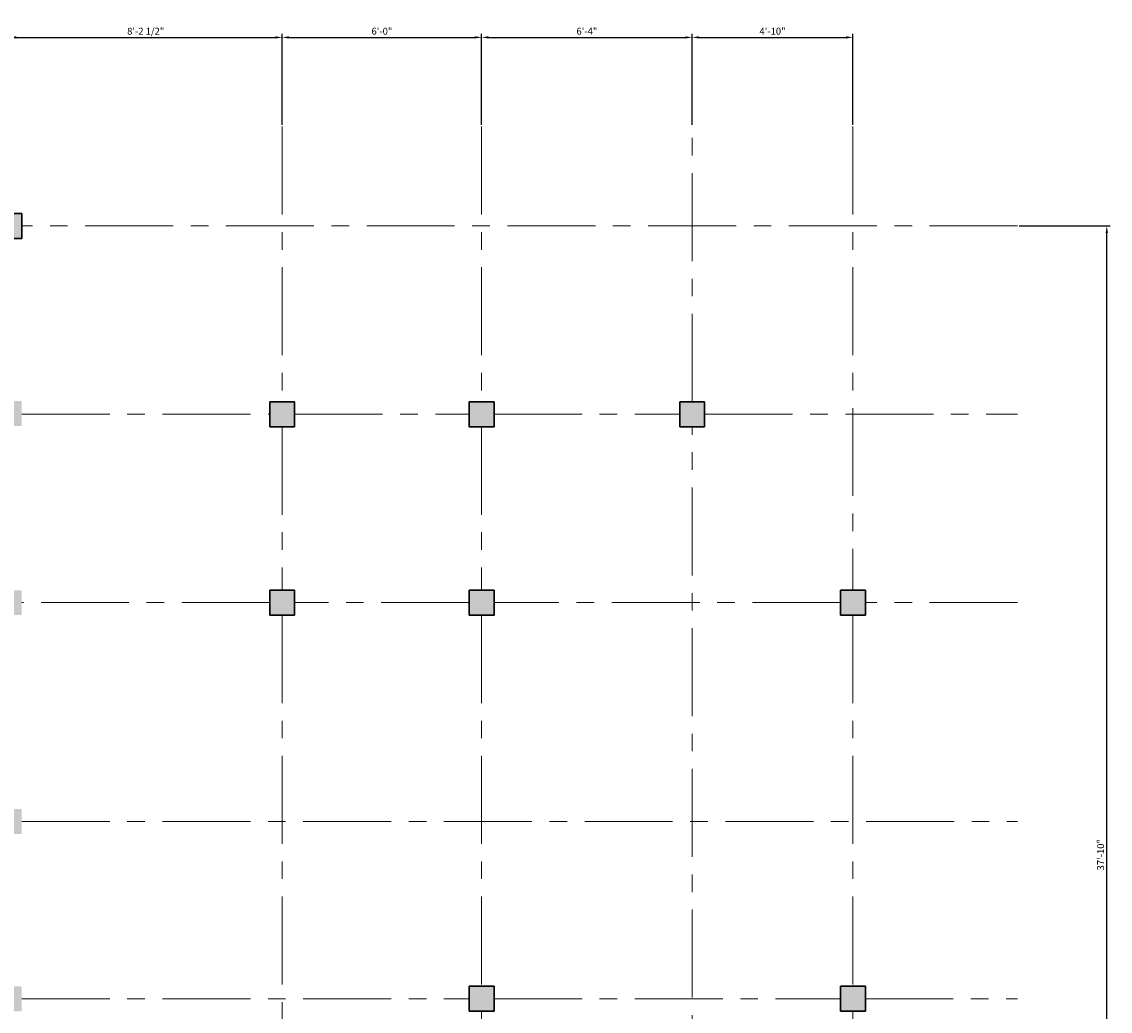
# Model space of a CAD drawing. Units: inches. Extents: x 4878 to 9282, y 5367 to 6617.
# Tile 9 of 14: x 5718 to 6111, y 6031 to 6388. Entities that reach past the tile are written whole.
import ezdxf

# ---------------------------------------------------------------- set-up
doc = ezdxf.new("R2010")
doc.units = ezdxf.units.IN
doc.linetypes.add('CENTER', pattern=[50.8, 31.75, -6.35, 6.35, -6.35])
for name, color, linetype, lineweight in [('A-ANNO-DIMS', 2, 'Continuous', 18), ('S-COLS', 1, 'Continuous', 30), ('S-COLS-PATT', 1, 'Continuous', 13), ('S-GRID', 4, 'CENTER', 13)]:
    doc.layers.add(name, color=color, linetype=linetype, lineweight=lineweight)
doc.styles.get("Standard").update_dxf_attribs({"font": 'arial.ttf'})
doc.dimstyles.new('ISO-25', dxfattribs={"dimtxt": 2.5, "dimasz": 2.5, "dimexe": 1.25, "dimexo": 0.625, "dimtad": 1, "dimdec": 0, "dimlunit": 3, "dimtxsty": 'Standard', "dimcen": 2.5, "dimadec": 0, "dimazin": 0, "dimtfac": 1, "dimtdec": 0, "dimtmove": 0, "dimatfit": 3, "dimfxl": 1, "dimarcsym": 0})

# ---------------------------------------------------------------- blocks, each defined once
blk = doc.blocks.new('COLUMN-9X9')
for p, q in [((0, 9), (9, 9)), ((0, 0), (0, 9)), ((9, 9), (9, 0)), ((0, 0), (9, 0))]:
    blk.add_line(p, q)
blk = doc.blocks.new('*D67')
at = {"layer": 'A-ANNO-DIMS', "color": 0, "lineweight": -2, "transparency": 16777216}
for p, q in [((5713.69, 6350.62), (5713.69, 6383.45)), ((5716.19, 6382.2), (5809.69, 6382.2)), ((5812.19, 6350.62), (5812.19, 6383.45))]:
    blk.add_line(p, q, dxfattribs=at)
at = {"layer": 'A-ANNO-DIMS', "color": 0, "transparency": 16777216}
for points in [[(5716.19, 6382.62), (5716.19, 6381.78), (5713.69, 6382.2)], [(5809.69, 6382.62), (5809.69, 6381.78), (5812.19, 6382.2)]]:
    blk.add_solid(points, dxfattribs=at)
at = {"layer": 'Defpoints', "color": 0, "transparency": 16777216}
for p in [(5812.19, 6382.2), (5713.69, 6350), (5812.19, 6350)]:
    blk.add_point(p, dxfattribs=at)
at = {"layer": 'A-ANNO-DIMS', "color": 0, "transparency": 16777216, "insert": (5762.94, 6384.12), "char_height": 2.5, "attachment_point": 5}
blk.add_mtext('8\'-2 1/2"', dxfattribs=at)
blk = doc.blocks.new('*D68')
at = {"layer": 'A-ANNO-DIMS', "color": 0, "lineweight": -2, "transparency": 16777216}
for p, q in [((5812.19, 6350.62), (5812.19, 6383.45)), ((5814.69, 6382.2), (5881.69, 6382.2)), ((5884.19, 6350.62), (5884.19, 6383.45))]:
    blk.add_line(p, q, dxfattribs=at)
at = {"layer": 'A-ANNO-DIMS', "color": 0, "transparency": 16777216}
for points in [[(5814.69, 6382.62), (5814.69, 6381.78), (5812.19, 6382.2)], [(5881.69, 6382.62), (5881.69, 6381.78), (5884.19, 6382.2)]]:
    blk.add_solid(points, dxfattribs=at)
at = {"layer": 'Defpoints', "color": 0, "transparency": 16777216}
for p in [(5884.19, 6382.2), (5812.19, 6350), (5884.19, 6350)]:
    blk.add_point(p, dxfattribs=at)
at = {"layer": 'A-ANNO-DIMS', "color": 0, "transparency": 16777216, "insert": (5848.19, 6384.1), "char_height": 2.5, "attachment_point": 5}
blk.add_mtext('6\'-0"', dxfattribs=at)
blk = doc.blocks.new('*D69')
at = {"layer": 'A-ANNO-DIMS', "color": 0, "lineweight": -2, "transparency": 16777216}
for p, q in [((5884.19, 6350.62), (5884.19, 6383.45)), ((5886.69, 6382.2), (5957.69, 6382.2)), ((5960.19, 6350.62), (5960.19, 6383.45))]:
    blk.add_line(p, q, dxfattribs=at)
at = {"layer": 'A-ANNO-DIMS', "color": 0, "transparency": 16777216}
for points in [[(5886.69, 6382.62), (5886.69, 6381.78), (5884.19, 6382.2)], [(5957.69, 6382.62), (5957.69, 6381.78), (5960.19, 6382.2)]]:
    blk.add_solid(points, dxfattribs=at)
at = {"layer": 'Defpoints', "color": 0, "transparency": 16777216}
for p in [(5960.19, 6382.2), (5884.19, 6350), (5960.19, 6350)]:
    blk.add_point(p, dxfattribs=at)
at = {"layer": 'A-ANNO-DIMS', "color": 0, "transparency": 16777216, "insert": (5922.19, 6384.1), "char_height": 2.5, "attachment_point": 5}
blk.add_mtext('6\'-4"', dxfattribs=at)
blk = doc.blocks.new('*D70')
at = {"layer": 'A-ANNO-DIMS', "color": 0, "lineweight": -2, "transparency": 16777216}
for p, q in [((5960.19, 6350.62), (5960.19, 6383.45)), ((5962.69, 6382.2), (6015.69, 6382.2)), ((6018.19, 6350.62), (6018.19, 6383.45))]:
    blk.add_line(p, q, dxfattribs=at)
at = {"layer": 'A-ANNO-DIMS', "color": 0, "transparency": 16777216}
for points in [[(5962.69, 6382.62), (5962.69, 6381.78), (5960.19, 6382.2)], [(6015.69, 6382.62), (6015.69, 6381.78), (6018.19, 6382.2)]]:
    blk.add_solid(points, dxfattribs=at)
at = {"layer": 'Defpoints', "color": 0, "transparency": 16777216}
for p in [(6018.19, 6382.2), (5960.19, 6350), (6018.19, 6350)]:
    blk.add_point(p, dxfattribs=at)
at = {"layer": 'A-ANNO-DIMS', "color": 0, "transparency": 16777216, "insert": (5989.19, 6384.1), "char_height": 2.5, "attachment_point": 5}
blk.add_mtext('4\'-10"', dxfattribs=at)
blk = doc.blocks.new('*D78')
at = {"layer": 'A-ANNO-DIMS', "color": 0, "lineweight": -2, "transparency": 16777216}
for p, q in [((6078.26, 6314.14), (6111.09, 6314.14)), ((6109.84, 5862.64), (6109.84, 6311.64)), ((6078.26, 5860.14), (6111.09, 5860.14))]:
    blk.add_line(p, q, dxfattribs=at)
at = {"layer": 'A-ANNO-DIMS', "color": 0, "transparency": 16777216}
for points in [[(6109.42, 6311.64), (6110.26, 6311.64), (6109.84, 6314.14)], [(6109.42, 5862.64), (6110.26, 5862.64), (6109.84, 5860.14)]]:
    blk.add_solid(points, dxfattribs=at)
at = {"layer": 'Defpoints', "color": 0, "transparency": 16777216}
for p in [(6077.64, 6314.14), (6109.84, 6314.14), (6077.64, 5860.14)]:
    blk.add_point(p, dxfattribs=at)
at = {"layer": 'A-ANNO-DIMS', "color": 0, "transparency": 16777216, "insert": (6107.94, 6087.14), "char_height": 2.5, "attachment_point": 5, "rotation": 90}
blk.add_mtext('37\'-10"', dxfattribs=at)

msp = doc.modelspace()

# ---------------------------------------------------------------- hatches: boundary and pattern name
at = {"layer": 'S-COLS-PATT'}
h = msp.add_hatch(color=256, dxfattribs=at)
h.dxf.hatch_style = 1
h.paths.add_polyline_path([(5621.19, 6309.64), (5630.19, 6309.64), (5630.19, 6318.64), (5621.19, 6318.64)])
h.paths.add_polyline_path([(5718.19, 6318.64), (5709.19, 6318.64), (5709.19, 6309.64), (5718.19, 6309.64)])
h.paths.add_polyline_path([(5575.19, 6241.64), (5575.19, 6250.64), (5566.19, 6250.64), (5566.19, 6241.64)])
h.paths.add_polyline_path([(5709.19, 6241.92), (5718.19, 6241.92), (5718.19, 6250.92), (5709.19, 6250.92)])
h.paths.add_polyline_path([(5816.69, 6250.64), (5807.69, 6250.64), (5807.69, 6241.64), (5816.69, 6241.64)])
h.paths.add_polyline_path([(5888.69, 6250.64), (5879.69, 6250.64), (5879.69, 6241.64), (5888.69, 6241.64)])
h.paths.add_polyline_path([(5964.69, 6250.64), (5955.69, 6250.64), (5955.69, 6241.64), (5964.69, 6241.64)])
h.paths.add_polyline_path([(5718.19, 6182.64), (5709.19, 6182.64), (5709.19, 6173.64), (5718.19, 6173.64)])
h.paths.add_polyline_path([(5816.69, 6182.64), (5807.69, 6182.64), (5807.69, 6173.64), (5816.69, 6173.64)])
h.paths.add_polyline_path([(5888.69, 6182.64), (5879.69, 6182.64), (5879.69, 6173.64), (5888.69, 6173.64)])
h.paths.add_polyline_path([(6013.69, 6173.64), (6022.69, 6173.64), (6022.69, 6182.64), (6013.69, 6182.64)])
h.paths.add_polyline_path([(6022.69, 6039.64), (6013.69, 6039.64), (6013.69, 6030.64), (6022.69, 6030.64)])
h.paths.add_polyline_path([(5879.69, 6030.64), (5888.69, 6030.64), (5888.69, 6039.64), (5879.69, 6039.64)])
h.paths.add_polyline_path([(5718.19, 6103.64), (5709.19, 6103.64), (5709.19, 6094.64), (5718.19, 6094.64)])
h.paths.add_polyline_path([(5718.19, 6039.64), (5709.19, 6039.64), (5709.19, 6030.64), (5718.19, 6030.64)])
h.paths.add_polyline_path([(5575.19, 6039.64), (5566.19, 6039.64), (5566.19, 6030.64), (5575.19, 6030.64)])
h.paths.add_polyline_path([(5566.19, 6094.64), (5575.19, 6094.64), (5575.19, 6103.64), (5566.19, 6103.64)])
h.paths.add_polyline_path([(5566.19, 5943.14), (5575.19, 5943.14), (5575.19, 5952.14), (5566.19, 5952.14)])
h.paths.add_polyline_path([(5575.19, 5864.64), (5566.19, 5864.64), (5566.19, 5855.64), (5575.19, 5855.64)])
h.paths.add_polyline_path([(5709.19, 5943.14), (5718.19, 5943.14), (5718.19, 5952.14), (5709.19, 5952.14)])
h.paths.add_polyline_path([(5718.19, 5855.64), (5718.19, 5864.64), (5709.19, 5864.64), (5709.19, 5855.64)])
h.paths.add_polyline_path([(5879.69, 5855.64), (5888.69, 5855.64), (5888.69, 5864.64), (5879.69, 5864.64)])
h.paths.add_polyline_path([(6013.69, 5855.64), (6022.69, 5855.64), (6022.69, 5864.64), (6013.69, 5864.64)])
h.paths.add_polyline_path([(5888.69, 5952.14), (5879.69, 5952.14), (5879.69, 5943.14), (5888.69, 5943.14)])

# ---------------------------------------------------------------- linework, layer by layer
at = {"layer": 'S-COLS'}
msp.add_line((5888.69, 6241.64), (5879.69, 6241.64), dxfattribs=at)
at = {"layer": 'S-GRID'}
for p, q in [((5812.19, 6350), (5812.19, 6250.64)), ((5884.19, 6350), (5884.19, 6250.64)), ((5960.19, 6250.64), (5960.19, 6350)), ((6018.19, 6350), (6018.19, 6182.64)), ((6077.64, 6314.14), (5718.19, 6314.14)), ((5718.19, 6246.14), (5807.69, 6246.14)), ((5816.69, 6246.14), (5879.69, 6246.14)), ((5888.69, 6246.14), (5955.69, 6246.14)), ((5964.69, 6246.14), (6077.64, 6246.14)), ((5812.19, 6241.64), (5812.19, 6182.64)), ((5884.19, 6241.64), (5884.19, 6182.64)), ((5960.19, 5781.57), (5960.19, 6241.64)), ((5807.69, 6178.14), (5718.19, 6178.14)), ((5879.69, 6178.14), (5816.69, 6178.14)), ((6013.69, 6178.14), (5888.69, 6178.14)), ((6077.64, 6178.14), (6022.69, 6178.14)), ((5812.19, 6173.64), (5812.19, 5781.04)), ((5884.19, 6173.64), (5884.19, 6039.64)), ((6018.19, 6173.64), (6018.19, 6039.64)), ((5718.19, 6099.14), (6077.64, 6099.14)), ((5718.19, 6035.14), (5879.69, 6035.14)), ((5888.69, 6035.14), (6013.69, 6035.14)), ((6022.69, 6035.14), (6077.64, 6035.14)), ((5884.19, 6030.64), (5884.19, 5952.14)), ((6018.19, 6030.64), (6018.19, 5864.64))]:
    msp.add_line(p, q, dxfattribs=at)

# ---------------------------------------------------------------- block references
at = {"layer": 'S-COLS'}
for p in [(5709.19, 6309.65), (5807.69, 6241.65), (5879.69, 6241.65), (5955.69, 6241.65), (5807.69, 6173.65), (5879.69, 6173.65), (6013.69, 6173.65), (5879.69, 6030.65), (6013.69, 6030.65)]:
    msp.add_blockref('COLUMN-9X9', p, dxfattribs=at)

# ---------------------------------------------------------------- dimensions: what is measured, and where the dimension line sits
at = {"layer": 'A-ANNO-DIMS'}
for base, p1, p2, picture, middle in [((5812.19, 6382.2), (5713.69, 6350), (5812.19, 6350), '*D67', (5762.94, 6384.12)), ((5884.19, 6382.2), (5812.19, 6350), (5884.19, 6350), '*D68', (5848.19, 6384.1)), ((5960.19, 6382.2), (5884.19, 6350), (5960.19, 6350), '*D69', (5922.19, 6384.1)), ((6018.19, 6382.2), (5960.19, 6350), (6018.19, 6350), '*D70', (5989.19, 6384.1))]:
    dim = msp.add_linear_dim(base=base, p1=p1, p2=p2, dimstyle='ISO-25', override={"dimdec": 1, "dimlfac": 1, "dimrnd": 0, "dimzin": 1, "dimdsep": 46, "dimlunit": 4, "dimfrac": 2}, dxfattribs=at)
    dim.commit()
    dim.dimension.update_dxf_attribs({"geometry": picture, "text_midpoint": middle})
dim = msp.add_linear_dim(base=(6109.84, 6314.14), p1=(6077.64, 5860.14), p2=(6077.64, 6314.14), angle=90, dimstyle='ISO-25', override={"dimdec": 1, "dimlfac": 1, "dimrnd": 0, "dimzin": 1, "dimdsep": 46, "dimlunit": 4, "dimfrac": 2}, dxfattribs=at)
dim.commit()
dim.dimension.update_dxf_attribs({"geometry": '*D78', "text_midpoint": (6107.94, 6087.14)})

doc.saveas('drawing.dxf')
